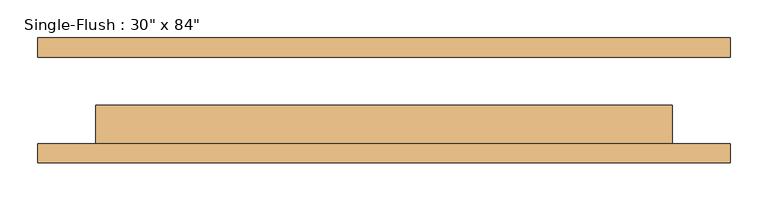
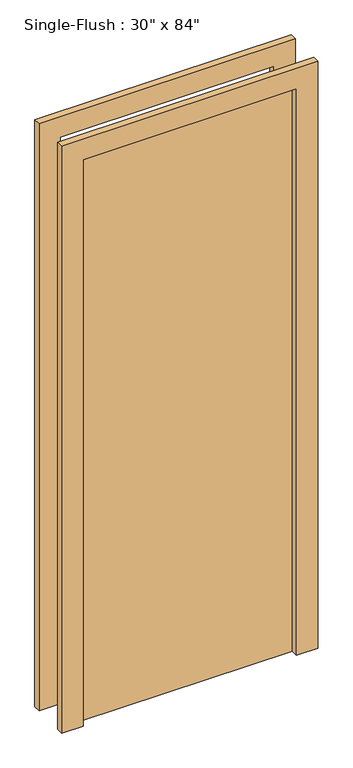
"""IFC4 building model written with IfcOpenShell, lengths in millimetres: door geometry."""

from ifc_helpers import new_model, si_unit, frame, origin, origin_with_axes, place, context, project, spatial, polyline, outline, extrude, source, transform, mapped, element, save


def door_78caadf7(model_context):
    return source(origin(), model_context, "Body", "SweptSolid", [
        extrude(outline(polyline([(2209.8, -457.2), (0.0, -457.2), (0.0, -381.0), (2133.6, -381.0), (2133.6, 381.0), (0.0, 381.0), (0.0, 457.2), (2209.8, 457.2), (2209.8, -457.2)])), frame((0.0, -82.55, 0.0), z_axis=(0.0, 1.0, 0.0), x_axis=(0.0, 0.0, 1.0)), (0.0, 0.0, 1.0), 25.4),
        extrude(outline(polyline([(2209.8, 457.2), (2209.8, -457.2), (0.0, -457.2), (0.0, -381.0), (2133.6, -381.0), (2133.6, 381.0), (0.0, 381.0), (0.0, 457.2), (2209.8, 457.2)])), frame((0.0, 57.15, 0.0), z_axis=(0.0, 1.0, 0.0), x_axis=(0.0, 0.0, 1.0)), (0.0, 0.0, 1.0), 25.4),
        extrude(outline(polyline([(381.0, -6.35), (381.0, -57.15), (-381.0, -57.15), (-381.0, -6.35), (381.0, -6.35)])), origin_with_axes(), (0.0, 0.0, 1.0), 2133.6),
    ])


if __name__ == "__main__":
    model = new_model("IFC4")
    model_context = context("Model", 3, world=origin())
    ifc_project = project(units=[si_unit("LENGTHUNIT", "METRE", prefix="MILLI")], contexts=[model_context])
    site = spatial("IfcSite", under=ifc_project)
    building = spatial("IfcBuilding", under=site)
    placement = place(None, origin())
    door_shape = door_78caadf7(model_context)
    element("IfcDoor", 1, ObjectType="Single-Flush : 30\" x 84\"", at=placement, inside=building, context=model_context, shape_type="MappedRepresentation", body=[
        mapped(door_shape, transform((0.0, 0.0, 0.0), x_axis=(1.0, 0.0, 0.0), y_axis=(0.0, 1.0, 0.0), z_axis=(0.0, 0.0, 1.0))),
    ])
    save(model, "model.ifc")

# Revit data of these elements
# Type "Single-Flush : 30\" x 84\""
#   Type Mark = "4"
#   Construction Type Id = "MDOOR"
#   Assembly Code = "C1020"
#   Analytic Construction = "Metal"
#   Thickness = 0' - 2"
#   Heat Transfer Coefficient (U) = 0.651978 BTU/(h·ft²·°F)
#   Height = 7' - 0"
#   Trim Projection Ext = 0' - 1"
#   Trim Projection Int = 0' - 1"
#   Trim Width = 0' - 3"
#   Width = 2' - 6"
#   Define Thermal Properties by = 1
#   Define Thermal Properties by = 1
#   Door Material = Door - Panel
#   Frame Material = Door - Frame
#   Visual Light Transmittance = 0
#   Solar Heat Gain Coefficient = 0
#   Function = (empty or 0)
#   Wall Closure = (empty or 0)
# Element 1 (IfcDoor, "Single-Flush : 30\" x 84\"")
#   Materials on its faces: "Door - Frame", "Door - Panel"
# Materials
#   "Door - Panel": class "Wood", colour RGB 210 159 95, transparency 0, Cost = 0
#   "Door - Frame": colour RGB 118 70 51, transparency 0, Cost = 0
